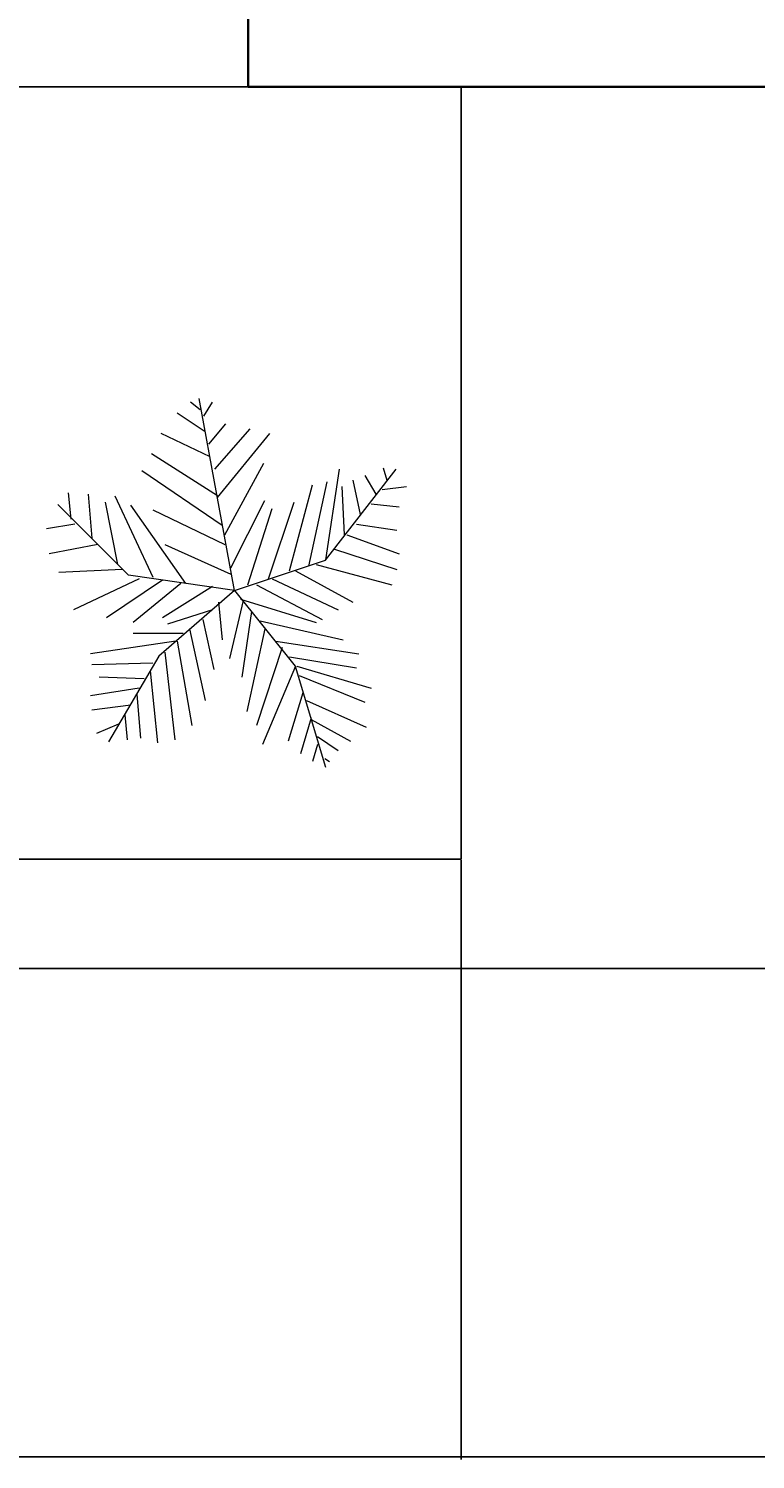
# Model space of a CAD drawing. Units: inches. Extents: x 4159 to 4826, y 299 to 1026.
# Tile 6 of 37: x 4354 to 4404, y 299 to 396. Entities that reach past the tile are written whole.
import ezdxf

# ---------------------------------------------------------------- set-up
doc = ezdxf.new("R2010")
doc.units = ezdxf.units.IN
for name, color, linetype, lineweight in [('A-ANNO-DIMS', 2, 'Continuous', 18), ('A-FLOR-BALC', 7, 'Continuous', 25), ('A-WALL', 7, 'Continuous', 35), ('L-PLNT', 94, 'Continuous', 13)]:
    doc.layers.add(name, color=color, linetype=linetype, lineweight=lineweight)
doc.styles.get("Standard").update_dxf_attribs({"font": 'arial.ttf'})
doc.dimstyles.get("Standard").update_dxf_attribs({"dimtxt": 0.18, "dimasz": 0.18, "dimexe": 0.18, "dimexo": 0.0625, "dimgap": 0.09, "dimtad": 0, "dimtih": 1, "dimtoh": 1, "dimdec": 4, "dimzin": 0, "dimdsep": 46, "dimtxsty": 'Standard', "dimcen": 0.09, "dimadec": 0, "dimazin": 0, "dimtfac": 1, "dimtdec": 4, "dimtofl": 0, "dimtmove": 0, "dimatfit": 3, "dimfxl": 1, "dimtolj": 1, "dimtzin": 0, "dimarcsym": 0})

# ---------------------------------------------------------------- blocks, each defined once
blk = doc.blocks.new('*U12')
for p, q in [((-10.186, 53.64), (-13.084, 55.962)), ((0, 0), (-10.5, 57)), ((-9.099, 51.782), (-6.563, 55.962)), ((-8.737, 47.138), (-17.069, 52.711)), ((-7.65, 43.423), (-2.578, 49.46)), ((-5.839, 35.992), (4.667, 48.067)), ((-7.288, 39.707), (-21.778, 46.673)), ((-5.114, 27.632), (10.463, 46.673)), ((-5.114, 28.097), (-24.676, 40.636)), ((-3.665, 19.273), (-27.574, 35.527)), ((-2.941, 16.486), (8.652, 37.85)), ((27, 9), (48, 36)), ((27.127, 9.056), (31.112, 35.992)), ((38.719, 34.134), (41.979, 28.561)), ((44.153, 36.456), (45.239, 32.741)), ((16.259, 5.805), (23.142, 31.348)), ((22.055, 7.198), (27.489, 32.277)), ((31.836, 30.883), (32.561, 16.486)), ((35.096, 32.741), (37.27, 22.524)), ((43.791, 29.954), (51.036, 30.883)), ((-48.585, 21.131), (-49.309, 29.026)), ((-43.513, 28.561), (-42.427, 15.558)), ((-38.442, 26.239), (-34.819, 7.663)), ((-35.544, 28.097), (-24.314, 3.947)), ((-1.129, 6.734), (9.014, 26.704)), ((10.101, 3.483), (17.708, 26.239)), ((40.53, 25.775), (48.862, 24.846)), ((-31.5, 4.5), (-52.5, 25.5)), ((-14.533, 2.09), (-30.834, 25.31)), ((-24.314, 23.917), (-2.941, 13.7)), ((3.942, 1.625), (11.187, 24.381)), ((-47.498, 19.737), (-55.83, 18.344)), ((36.183, 19.737), (48.137, 17.88)), ((-40.615, 13.7), (-55.105, 10.913)), ((-20.691, 13.7), (-1.129, 4.876)), ((33.285, 16.486), (48.862, 10.913)), ((0, 0), (27, 9)), ((29.662, 12.307), (48.137, 6.269)), ((-33.37, 6.269), (-52.207, 5.34)), ((0, 0), (-31.5, 4.5)), ((18.07, 5.805), (35.096, -3.483)), ((24.229, 7.663), (46.688, 1.625)), ((-28.299, 3.483), (-47.86, -5.805)), ((-21.416, 3.018), (-38.079, -8.128)), ((-15.982, 2.09), (-30.11, -9.521)), ((0, 0), (-22.5, -19.5)), ((-6.563, 1.161), (-21.416, -8.128)), ((0, 0), (18, -22.5)), ((6.478, 1.625), (26.04, -8.592)), ((11.187, 3.483), (30.749, -5.805)), ((-4.752, -3.483), (-3.665, -14.629)), ((2.493, -3.019), (-1.491, -20.202)), ((1.769, -2.555), (24.229, -9.521)), ((-6.563, -5.805), (-19.967, -9.985)), ((5.029, -6.27), (2.131, -25.775)), ((-13.446, -11.378), (-8.737, -32.741)), ((-9.461, -8.592), (-6.201, -23.453)), ((9.014, -11.378), (3.58, -35.992)), ((7.565, -9.056), (32.198, -14.629)), ((-17.431, -15.094), (-42.789, -18.809)), ((-15.257, -12.772), (-30.11, -12.772)), ((-17.069, -15.094), (-12.721, -40.172)), ((14.085, -16.951), (6.478, -40.172)), ((12.274, -15.094), (36.907, -18.809)), ((-22.5, -19.5), (-37.5, -45)), ((-20.691, -18.345), (-17.793, -44.352)), ((16.259, -19.738), (36.183, -22.989)), ((-24.314, -21.596), (-42.427, -22.06)), ((-25.038, -23.918), (-22.865, -45.281)), ((18.07, -22.524), (8.289, -45.745)), ((18, -22.5), (27, -52.5)), ((18.433, -22.524), (40.53, -29.026)), ((19.157, -25.311), (38.719, -33.206)), ((-28.299, -29.026), (-42.789, -31.348)), ((-26.849, -26.24), (-40.253, -25.775)), ((-29.023, -30.884), (-27.936, -43.887)), ((20.244, -30.419), (15.897, -44.816)), ((21.331, -32.741), (39.081, -40.636)), ((-30.834, -34.135), (-42.427, -35.528)), ((-32.646, -36.921), (-31.921, -44.352)), ((22.78, -37.85), (19.519, -48.532)), ((-34.457, -39.708), (-40.978, -42.494)), ((22.78, -38.314), (34.372, -44.816)), ((24.591, -45.745), (23.142, -50.854)), ((24.591, -43.423), (30.749, -47.603)), ((26.764, -49.925), (28.213, -50.854))]:
    blk.add_line(p, q)
blk = doc.blocks.new('*D44')
at = {"layer": 'A-ANNO-DIMS', "color": 0, "lineweight": -2, "transparency": 16777216}
for p, q in [((4287.263, 963.093), (4158.88, 963.093)), ((4159.06, 962.913), (4159.06, 647.826)), ((4159.06, 332.375), (4159.06, 647.462)), ((4447.248, 332.195), (4158.88, 332.195))]:
    blk.add_line(p, q, dxfattribs=at)
at = {"layer": 'A-ANNO-DIMS', "color": 0, "transparency": 16777216}
for points in [[(4159.03, 962.913), (4159.09, 962.913), (4159.06, 963.093)], [(4159.03, 332.375), (4159.09, 332.375), (4159.06, 332.195)]]:
    blk.add_solid(points, dxfattribs=at)
at = {"layer": 'Defpoints', "color": 0, "transparency": 16777216}
for p in [(4287.326, 963.093), (4159.06, 332.195), (4447.31, 332.195)]:
    blk.add_point(p, dxfattribs=at)
at = {"layer": 'A-ANNO-DIMS', "color": 0, "transparency": 16777216, "insert": (4159.06, 647.644), "char_height": 0.18, "attachment_point": 5}
blk.add_mtext('\\A1;630.9', dxfattribs=at)
blk = doc.blocks.new('*D46')
at = {"layer": 'A-ANNO-DIMS', "color": 0, "lineweight": -2, "transparency": 16777216}
for p, q in [((4192.31, 392.192), (4192.31, 298.765)), ((4447.31, 332.133), (4447.31, 298.765)), ((4192.49, 298.945), (4319.519, 298.945)), ((4447.13, 298.945), (4320.101, 298.945))]:
    blk.add_line(p, q, dxfattribs=at)
at = {"layer": 'A-ANNO-DIMS', "color": 0, "transparency": 16777216}
for points in [[(4192.49, 298.975), (4192.49, 298.915), (4192.31, 298.945)], [(4447.13, 298.975), (4447.13, 298.915), (4447.31, 298.945)]]:
    blk.add_solid(points, dxfattribs=at)
at = {"layer": 'Defpoints', "color": 0, "transparency": 16777216}
for p in [(4192.31, 392.254), (4447.31, 332.195), (4447.31, 298.945)]:
    blk.add_point(p, dxfattribs=at)
at = {"layer": 'A-ANNO-DIMS', "color": 0, "transparency": 16777216, "insert": (4319.81, 298.945), "char_height": 0.18, "attachment_point": 5}
blk.add_mtext('\\A1;255', dxfattribs=at)
blk = doc.blocks.new('*D53')
at = {"layer": 'A-ANNO-DIMS', "color": 0, "lineweight": -2, "transparency": 16777216}
for p, q in [((4267.89, 339.581), (4267.89, 298.765)), ((4383.821, 339.581), (4383.821, 298.765)), ((4268.07, 298.945), (4325.4, 298.945)), ((4383.641, 298.945), (4326.311, 298.945))]:
    blk.add_line(p, q, dxfattribs=at)
at = {"layer": 'A-ANNO-DIMS', "color": 0, "transparency": 16777216}
for points in [[(4268.07, 298.975), (4268.07, 298.915), (4267.89, 298.945)], [(4383.641, 298.975), (4383.641, 298.915), (4383.821, 298.945)]]:
    blk.add_solid(points, dxfattribs=at)
at = {"layer": 'Defpoints', "color": 0, "transparency": 16777216}
for p in [(4267.89, 339.644), (4383.821, 339.644), (4383.821, 298.945)]:
    blk.add_point(p, dxfattribs=at)
at = {"layer": 'A-ANNO-DIMS', "color": 0, "transparency": 16777216, "insert": (4325.855, 298.945), "char_height": 0.18, "attachment_point": 5}
blk.add_mtext('\\A1;115.93', dxfattribs=at)

msp = doc.modelspace()

# ---------------------------------------------------------------- linework, layer by layer
at = {"layer": 'A-FLOR-BALC'}
msp.add_lwpolyline([(4267.89, 392.254), (4383.821, 392.254), (4383.821, 339.644), (4267.89, 339.644)], close=True, dxfattribs=at)
at = {"layer": 'A-WALL'}
for p in [(4369.31, 401.254), (4447.31, 392.254)]:
    msp.add_line(p, (4369.31, 392.254), dxfattribs=at)

# ---------------------------------------------------------------- block references
at = {"layer": 'L-PLNT', "xscale": 0.2292012274639507, "yscale": 0.2292012274639507, "zscale": 0.2292012274639507}
msp.add_blockref('*U12', (4368.395, 357.945), dxfattribs=at)

# ---------------------------------------------------------------- dimensions: what is measured, and where the dimension line sits
at = {"layer": 'A-ANNO-DIMS'}
dim = msp.add_linear_dim(base=(4159.06, 332.195), p1=(4287.326, 963.093), p2=(4447.31, 332.195), angle=90, dimstyle='Standard', override={"dimdec": 1, "dimlfac": 1, "dimrnd": 0, "dimzin": 0, "dimdsep": 46, "dimlunit": 2}, dxfattribs=at)
dim.commit()
dim.dimension.update_dxf_attribs({"geometry": '*D44', "text_midpoint": (4159.06, 647.644)})
for base, p1, p2, override, picture, middle in [((4447.31, 298.945), (4192.31, 392.254), (4447.31, 332.195), {"dimdec": 0, "dimlfac": 1, "dimrnd": 0, "dimzin": 0, "dimdsep": 46, "dimlunit": 2}, '*D46', (4319.81, 298.945)), ((4383.821, 298.945), (4267.89, 339.644), (4383.821, 339.644), {"dimdec": 2, "dimlfac": 1, "dimrnd": 0, "dimzin": 0, "dimdsep": 46, "dimlunit": 2}, '*D53', (4325.855, 298.945))]:
    dim = msp.add_linear_dim(base=base, p1=p1, p2=p2, dimstyle='Standard', override=override, dxfattribs=at)
    dim.commit()
    dim.dimension.update_dxf_attribs({"geometry": picture, "text_midpoint": middle})

doc.saveas('drawing.dxf')
